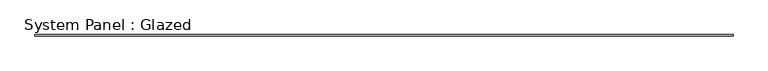
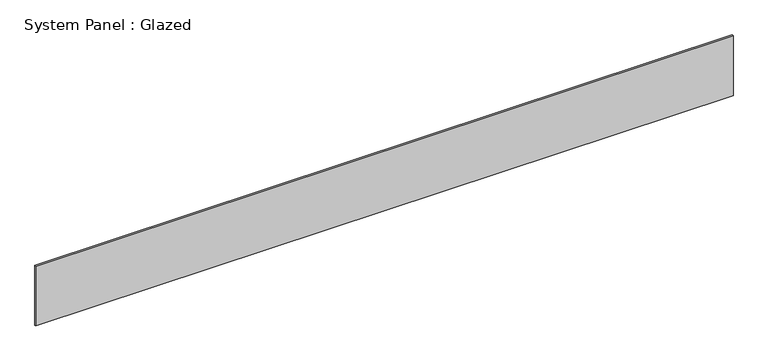
"""IFC4 building model written with IfcOpenShell, lengths in millimetres: plate geometry, System Panel : Glazed."""

from ifc_helpers import new_model, si_unit, origin, origin_with_axes, place, context, project, spatial, polyline, outline, extrude, source, transform, mapped, element, save


def system_panel_glazed_d9f0472a(model_context):
    return source(origin(), model_context, "Body", "SweptSolid", [
        extrude(outline(polyline([(6369.4891855, 19.05), (-6369.4891855, 19.05), (-6369.4891855, 44.45), (6369.4891855, 44.45), (6369.4891855, 19.05)])), origin_with_axes(), (0.0, 0.0, 1.0), 1155.7),
    ])


if __name__ == "__main__":
    model = new_model("IFC4")
    model_context = context("Model", 3, world=origin())
    ifc_project = project(units=[si_unit("LENGTHUNIT", "METRE", prefix="MILLI")], contexts=[model_context])
    site = spatial("IfcSite", under=ifc_project)
    building = spatial("IfcBuilding", under=site)
    placement = place(None, origin())
    system_panel_glazed_shape = system_panel_glazed_d9f0472a(model_context)
    element("IfcPlate", 1, ObjectType="System Panel : Glazed", at=placement, inside=building, context=model_context, shape_type="MappedRepresentation", body=[
        mapped(system_panel_glazed_shape, transform((0.0, 0.0, 0.0), x_axis=(1.0, 0.0, 0.0), y_axis=(0.0, 1.0, 0.0), z_axis=(0.0, 0.0, 1.0))),
    ])
    save(model, "model.ifc")

# Revit data of these elements
# Type "System Panel : Glazed"
#   Construction Type Id = "GSP4R"
#   Analytic Construction = "1/8 in Pilkington single glazing"
#   Visual Light Transmittance = 0.9
#   Solar Heat Gain Coefficient = 0.86
#   Heat Transfer Coefficient (U) = 1.18115 BTU/(h·ft²·°F)
# Element 1 (IfcPlate, "System Panel : Glazed")
#   Materials on its faces: "Glass"
# Materials
#   "Glass": class "Glass", colour RGB 0 128 192, transparency 0.75, Description = "Soda Lime Glass", Cost = 0
